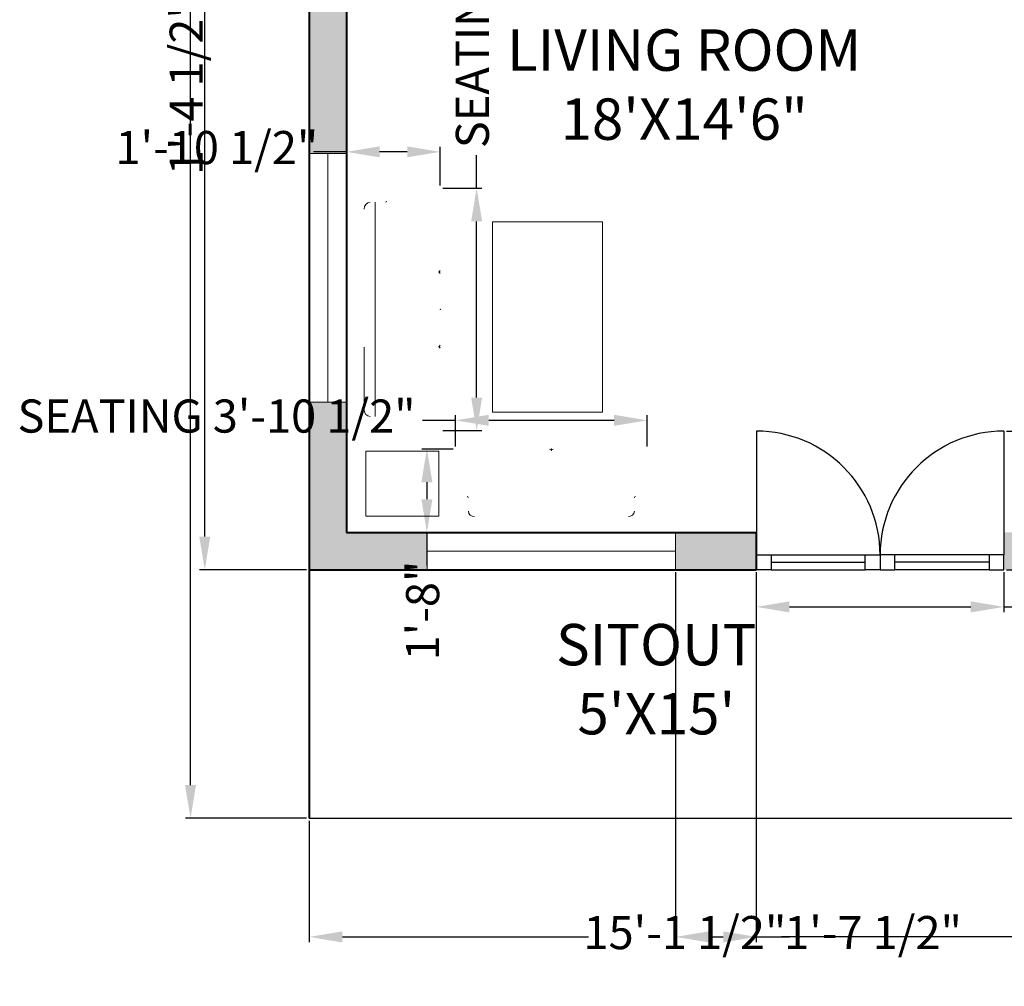
# Model space of a CAD drawing. Units: inches. Extents: x 2138 to 3265, y 2149 to 3392.
# Tile 1 of 13: x 2138 to 2375, y 2149 to 2382. Entities that reach past the tile are written whole.
import ezdxf

# ---------------------------------------------------------------- set-up
doc = ezdxf.new("R2010")
doc.units = ezdxf.units.IN
for name, color, linetype, lineweight in [('A-ANNO-DIMS', 2, 'Continuous', 18), ('A-AREA-IDEN', 7, 'Continuous', 18), ('A-DOOR', 22, 'Continuous', 25), ('A-FLOR', 7, 'Continuous', 25), ('A-FURN', 8, 'Continuous', 18), ('A-GLAZ', 150, 'Continuous', 18), ('A-WALL', 7, 'Continuous', 40), ('A-WALL-PATT', 142, 'Continuous', 13)]:
    doc.layers.add(name, color=color, linetype=linetype, lineweight=lineweight)
doc.styles.get("Standard").update_dxf_attribs({"font": 'arial.ttf'})
doc.dimstyles.new('ISO-25', dxfattribs={"dimtxt": 8, "dimasz": 8, "dimexe": 1.25, "dimexo": 0.625, "dimtad": 0, "dimdec": 1, "dimlunit": 4, "dimtxsty": 'Standard', "dimcen": 2.5, "dimadec": 0, "dimazin": 0, "dimtfac": 1, "dimtdec": 1, "dimtmove": 0, "dimatfit": 3, "dimfxl": 1, "dimarcsym": 0})

# ---------------------------------------------------------------- blocks, each defined once
blk = doc.blocks.new('Clinicians and patient chairs 13_dwgmodels.com')
at = {"color": 0}
for points in [[(-780.9, 0, 0, 0, 0), (-832.6, -11.1, 4.5, 4.5, 0)], [(-780.8, -0.7, 0, 0, 0), (-832.3, -11.8, 4.5, 4.5, 0)], [(-780.8, -0.7, 0, 0, 0), (-832.3, -11.8, 4.5, 4.5, 0)], [(780.9, 0, 0, 0, 0), (-780.9, 0, 4.5, 4.5, 0)], [(780.8, -0.7, 0, 0, 0), (-780.8, -0.7, 4.5, 4.5, 0)], [(780.8, -0.7, 0, 0, 0), (-780.8, -0.7, 4.5, 4.5, 0)], [(832.3, -11.8, 0, 0, 0), (780.8, -0.7, 4.5, 4.5, 0)], [(832.3, -11.8, 0, 0, 0), (780.8, -0.7, 4.5, 4.5, 0)], [(832.6, -11.1, 0, 0, 0), (780.9, 0, 4.5, 4.5, 0)], [(-888.6, -68.3, 0, 0, 0), (-898.5, -106.3, 4.5, 4.5, 0)], [(-888, -68.6, 0, 0, 0), (-897.8, -106.4, 4.5, 4.5, 0)], [(-867.7, -35.9, 0, 0, 0), (-888.6, -68.3, 4.5, 4.5, 0)], [(-867.1, -36.4, 0, 0, 0), (-888, -68.6, 4.5, 4.5, 0)], [(-867.1, -36.4, 0, 0, 0), (-888, -68.6, 4.5, 4.5, 0)], [(-872.1, -47.4, 0, 0, 0), (-872.1, -47.3, 4.5, 4.5, 0)], [(-832.6, -11.1, 0, 0, 0), (-867.7, -35.9, 4.5, 4.5, 0)], [(-832.3, -11.8, 0, 0, 0), (-867.1, -36.4, 4.5, 4.5, 0)], [(-832.3, -11.8, 0, 0, 0), (-867.1, -36.4, 4.5, 4.5, 0)], [(-854.1, -29.4, 0, 0, 0), (-854.1, -29.4, 4.5, 4.5, 0)], [(867.1, -36.4, 0, 0, 0), (832.3, -11.8, 4.5, 4.5, 0)], [(867.1, -36.4, 0, 0, 0), (832.3, -11.8, 4.5, 4.5, 0)], [(867.7, -35.9, 0, 0, 0), (832.6, -11.1, 4.5, 4.5, 0)], [(888, -68.6, 0, 0, 0), (867.1, -36.4, 4.5, 4.5, 0)], [(888, -68.6, 0, 0, 0), (867.1, -36.4, 4.5, 4.5, 0)], [(888.6, -68.3, 0, 0, 0), (867.7, -35.9, 4.5, 4.5, 0)], [(897.8, -106.4, 0, 0, 0), (888, -68.6, 4.5, 4.5, 0)], [(897.8, -106.4, 0, 0, 0), (888, -68.6, 4.5, 4.5, 0)], [(898.5, -106.3, 0, 0, 0), (888.6, -68.3, 4.5, 4.5, 0)], [(-898.5, -106.3, 0, 0, 0), (-898.5, -766.8, 4.5, 4.5, 0)], [(-897.8, -106.4, 0, 0, 0), (-897.8, -114.4, 4.5, 4.5, 0)], [(-897.8, -106.4, 0, 0, 0), (-897.8, -114.4, 4.5, 4.5, 0)], [(-897.8, -114.4, 0, 0, 0), (-897.8, -766.7, 4.5, 4.5, 0)], [(-897.8, -114.4, 0, 0, 0), (-897.8, -766.7, 4.5, 4.5, 0)], [(-897.8, -766.7, 0, 0, 0), (-897.8, -114.4, 4.5, 4.5, 0)], [(-896, -117.6, 0, 0, 0), (-896, -126.8, 4.5, 4.5, 0)], [(-896, -117.6, 0, 0, 0), (-896, -324.6, 4.5, 4.5, 0)], [(-896, -126.8, 0, 0, 0), (-896, -324.6, 4.5, 4.5, 0)], [(-22.2, -148.3, 0, 0, 0), (-722.5, -148.3, 4.5, 4.5, 0)], [(-8.3, -148.3, 0, 0, 0), (-22.2, -148.3, 4.5, 4.5, 0)], [(-8.3, -148.3, 0, 0, 0), (-7.7, -148.3, 4.5, 4.5, 0)], [(-7.7, -148.3, 0, 0, 0), (-6.2, -148.3, 4.5, 4.5, 0)], [(-6.2, -148.3, 0, 0, 0), (-1.3, -150.4, 4.5, 4.5, 0)], [(2.3, -149.9, 0, 0, 0), (-2.3, -149.9, 4.5, 4.5, 0)], [(-1.3, -150.4, 0, 0, 0), (0, -159.3, 4.5, 4.5, 0)], [(1.3, -150.4, 0, 0, 0), (0, -159.3, 4.5, 4.5, 0)], [(0, -159.3, 0, 0, 0), (0, -764.6, 4.5, 4.5, 0)], [(0, -159.3, 0, 0, 0), (0, -764.6, 4.5, 4.5, 0)], [(6.2, -148.3, 0, 0, 0), (1.3, -150.4, 4.5, 4.5, 0)], [(7.7, -148.3, 0, 0, 0), (6.2, -148.3, 4.5, 4.5, 0)], [(8.3, -148.3, 0, 0, 0), (7.7, -148.3, 4.5, 4.5, 0)], [(22.2, -148.3, 0, 0, 0), (8.3, -148.3, 4.5, 4.5, 0)], [(206.6, -148.3, 0, 0, 0), (22.2, -148.3, 4.5, 4.5, 0)], [(206.6, -148.3, 0, 0, 0), (722.5, -148.3, 4.5, 4.5, 0)], [(897.8, -114.4, 0, 0, 0), (897.8, -106.4, 4.5, 4.5, 0)], [(897.8, -114.4, 0, 0, 0), (897.8, -106.4, 4.5, 4.5, 0)], [(897.8, -766.7, 0, 0, 0), (897.8, -114.4, 4.5, 4.5, 0)], [(898.5, -766.8, 0, 0, 0), (898.5, -106.3, 4.5, 4.5, 0)], [(898.5, -766.8, 0, 0, 0), (898.5, -117.3, 4.5, 4.5, 0)], [(-896, -321.9, 0, 0, 0), (-896, -251.5, 4.5, 4.5, 0)], [(-779.6, -285, 0, 0, 0), (-779.4, -198.1, 4.5, 4.5, 0)], [(779.6, -285, 0, 0, 0), (779.4, -198.1, 4.5, 4.5, 0)], [(-896, -317.7, 0, 0, 0), (-896, -329.7, 4.5, 4.5, 0)], [(-896, -320.4, 0, 0, 0), (-896, -324.6, 4.5, 4.5, 0)], [(-896, -321.9, 0, 0, 0), (-896, -329.7, 4.5, 4.5, 0)], [(-896, -329.7, 0, 0, 0), (-896, -321.9, 4.5, 4.5, 0)], [(-896, -329.7, 0, 0, 0), (-892.2, -332.9, 4.5, 4.5, 0)], [(-892.2, -332.9, 0, 0, 0), (-892, -333, 4.5, 4.5, 0)], [(-892, -333, 0, 0, 0), (-891.9, -333.1, 4.5, 4.5, 0)], [(-886.9, -334.2, 0, 0, 0), (-891.9, -333.1, 4.5, 4.5, 0)], [(-886.9, -334.2, 0, 0, 0), (-837.4, -335.7, 4.5, 4.5, 0)], [(-837.4, -335.7, 0, 0, 0), (-790.1, -337, 4.5, 4.5, 0)], [(-779.8, -305.4, 0, 0, 0), (-779.9, -324.5, 4.5, 4.5, 0)], [(-779.6, -285, 0, 0, 0), (-779.8, -305.4, 4.5, 4.5, 0)], [(779.6, -285, 0, 0, 0), (779.8, -305.4, 4.5, 4.5, 0)], [(779.8, -305.4, 0, 0, 0), (779.9, -324.5, 4.5, 4.5, 0)], [(837.4, -335.7, 0, 0, 0), (790.1, -337, 4.5, 4.5, 0)], [(886.9, -334.2, 0, 0, 0), (837.4, -335.7, 4.5, 4.5, 0)], [(886.9, -334.2, 0, 0, 0), (891.9, -333.1, 4.5, 4.5, 0)], [(891.9, -333.1, 0, 0, 0), (892, -333, 4.5, 4.5, 0)], [(892.2, -332.9, 0, 0, 0), (892, -333, 4.5, 4.5, 0)], [(896, -329.7, 0, 0, 0), (892.2, -332.9, 4.5, 4.5, 0)], [(-898.5, -766.8, 0, 0, 0), (-895.2, -776, 4.5, 4.5, 0)], [(-895.2, -776, 0, 0, 0), (-898.5, -766.8, 4.5, 4.5, 0)], [(-897.8, -766.7, 0, 0, 0), (-894.5, -775.7, 4.5, 4.5, 0)], [(-897.8, -766.7, 0, 0, 0), (-894.5, -775.7, 4.5, 4.5, 0)], [(-894.5, -775.7, 0, 0, 0), (-897.8, -766.7, 4.5, 4.5, 0)], [(-894.5, -775.7, 0, 0, 0), (-897.8, -766.7, 4.5, 4.5, 0)], [(-895.2, -776, 0, 0, 0), (-894.6, -777.1, 4.5, 4.5, 0)], [(-894.6, -777.1, 0, 0, 0), (-895.2, -776, 4.5, 4.5, 0)], [(-894.5, -775.7, 0, 0, 0), (-894, -776.6, 4.5, 4.5, 0)], [(-894.5, -775.7, 0, 0, 0), (-894, -776.6, 4.5, 4.5, 0)], [(-894, -776.6, 0, 0, 0), (-894.5, -775.7, 4.5, 4.5, 0)], [(-894, -776.6, 0, 0, 0), (-894.5, -775.7, 4.5, 4.5, 0)], [(-894.6, -777.1, 0, 0, 0), (-893.6, -777.8, 4.5, 4.5, 0)], [(-893.6, -777.8, 0, 0, 0), (-894.6, -777.1, 4.5, 4.5, 0)], [(-894, -776.6, 0, 0, 0), (-893.2, -777.2, 4.5, 4.5, 0)], [(-894, -776.6, 0, 0, 0), (-893.2, -777.2, 4.5, 4.5, 0)], [(-893.2, -777.2, 0, 0, 0), (-894, -776.6, 4.5, 4.5, 0)], [(-893.2, -777.2, 0, 0, 0), (-894, -776.6, 4.5, 4.5, 0)], [(-893.6, -777.8, 0, 0, 0), (-886.6, -781, 4.5, 4.5, 0)], [(-886.6, -781, 0, 0, 0), (-893.6, -777.8, 4.5, 4.5, 0)], [(-893.2, -777.2, 0, 0, 0), (-886.5, -780.3, 4.5, 4.5, 0)], [(-893.2, -777.2, 0, 0, 0), (-886.5, -780.3, 4.5, 4.5, 0)], [(-886.5, -780.3, 0, 0, 0), (-893.2, -777.2, 4.5, 4.5, 0)], [(-886.5, -780.3, 0, 0, 0), (-893.2, -777.2, 4.5, 4.5, 0)], [(-886.6, -781, 0, 0, 0), (886.6, -781, 4.5, 4.5, 0)], [(886.6, -781, 0, 0, 0), (-886.6, -781, 4.5, 4.5, 0)], [(-886.5, -780.3, 0, 0, 0), (886.5, -780.3, 4.5, 4.5, 0)], [(-886.5, -780.3, 0, 0, 0), (886.5, -780.3, 4.5, 4.5, 0)], [(886.5, -780.3, 0, 0, 0), (-886.5, -780.3, 4.5, 4.5, 0)], [(886.5, -780.3, 0, 0, 0), (-886.5, -780.3, 4.5, 4.5, 0)], [(886.5, -780.3, 0, 0, 0), (893.2, -777.2, 4.5, 4.5, 0)], [(886.5, -780.3, 0, 0, 0), (893.2, -777.2, 4.5, 4.5, 0)], [(893.2, -777.2, 0, 0, 0), (886.5, -780.3, 4.5, 4.5, 0)], [(893.2, -777.2, 0, 0, 0), (886.5, -780.3, 4.5, 4.5, 0)], [(886.6, -781, 0, 0, 0), (893.6, -777.8, 4.5, 4.5, 0)], [(893.6, -777.8, 0, 0, 0), (886.6, -781, 4.5, 4.5, 0)], [(893.2, -777.2, 0, 0, 0), (894, -776.6, 4.5, 4.5, 0)], [(893.2, -777.2, 0, 0, 0), (894, -776.6, 4.5, 4.5, 0)], [(894, -776.6, 0, 0, 0), (893.2, -777.2, 4.5, 4.5, 0)], [(894, -776.6, 0, 0, 0), (893.2, -777.2, 4.5, 4.5, 0)], [(893.6, -777.8, 0, 0, 0), (894.6, -777.1, 4.5, 4.5, 0)], [(894.6, -777.1, 0, 0, 0), (893.6, -777.8, 4.5, 4.5, 0)], [(894.5, -775.7, 0, 0, 0), (894, -776.6, 4.5, 4.5, 0)], [(894.5, -775.7, 0, 0, 0), (894, -776.6, 4.5, 4.5, 0)], [(894.5, -775.7, 0, 0, 0), (894, -776.6, 4.5, 4.5, 0)], [(894.5, -775.7, 0, 0, 0), (894, -776.6, 4.5, 4.5, 0)], [(894.5, -775.7, 0, 0, 0), (897.8, -766.7, 4.5, 4.5, 0)], [(894.5, -775.7, 0, 0, 0), (897.8, -766.7, 4.5, 4.5, 0)], [(897.8, -766.7, 0, 0, 0), (894.5, -775.7, 4.5, 4.5, 0)], [(897.8, -766.7, 0, 0, 0), (894.5, -775.7, 4.5, 4.5, 0)], [(895.2, -776, 0, 0, 0), (894.6, -777.1, 4.5, 4.5, 0)], [(895.2, -776, 0, 0, 0), (894.6, -777.1, 4.5, 4.5, 0)], [(895.2, -776, 0, 0, 0), (898.5, -766.8, 4.5, 4.5, 0)], [(898.5, -766.8, 0, 0, 0), (895.2, -776, 4.5, 4.5, 0)]]:
    blk.add_lwpolyline(points, format="xyseb", dxfattribs=at)
for points in [[(-779.9, -324.5), (-779.9, -328.3)], [(779.9, -324.5), (779.9, -325.8)]]:
    blk.add_lwpolyline(points, dxfattribs=at)
for centre, radius, start, end in [((-724.7, -203.1), 54.9, 87.66786, 174.72548), ((724.7, -203.1), 54.9, 5.27444, 92.33206), ((-789.7, -327.1), 9.9, 267.95505, 352.93087), ((791.8, -325.1), 12, 183.2786, 261.48612), ((-17.2, -763), 17.3, 271.1045, 354.62389), ((17.2, -763), 17.3, 185.37611, 268.8955)]:
    blk.add_arc(centre, radius, start, end, dxfattribs=at)
blk.add_point((0, -781), dxfattribs=at)
blk = doc.blocks.new('Clinicians and patient chairs 9_dwgmodels.com')
at = {"color": 0}
for points in [[(-907.9, 0, 0, 0, 0), (-959.6, -11.1, 4.62, 4.62, 0)], [(907.9, 0, 0, 0, 0), (-907.9, 0, 4.62, 4.62, 0)], [(959.6, -11.1, 0, 0, 0), (907.9, 0, 4.62, 4.62, 0)], [(-1015.6, -68.3, 0, 0, 0), (-1025.5, -106.3, 4.62, 4.62, 0)], [(-994.7, -35.9, 0, 0, 0), (-1015.6, -68.3, 4.62, 4.62, 0)], [(-959.6, -11.1, 0, 0, 0), (-994.7, -35.9, 4.62, 4.62, 0)], [(994.7, -35.9, 0, 0, 0), (959.6, -11.1, 4.62, 4.62, 0)], [(1015.6, -68.3, 0, 0, 0), (994.7, -35.9, 4.62, 4.62, 0)], [(1025.5, -106.3, 0, 0, 0), (1015.6, -68.3, 4.62, 4.62, 0)], [(-1025.5, -106.3, 0, 0, 0), (-1025.5, -779.5, 4.62, 4.62, 0)], [(-313.4, -149.9, 0, 0, 0), (-318.1, -149.9, 4.62, 4.62, 0)], [(-314.5, -150.4, 0, 0, 0), (-315.7, -159.3, 4.62, 4.62, 0)], [(-315.7, -159.3, 0, 0, 0), (-315.7, -777.3, 4.62, 4.62, 0)], [(-309.5, -148.3, 0, 0, 0), (-314.5, -150.4, 4.62, 4.62, 0)], [(-308, -148.3, 0, 0, 0), (-309.5, -148.3, 4.62, 4.62, 0)], [(-307.5, -148.3, 0, 0, 0), (-308, -148.3, 4.62, 4.62, 0)], [(242.9, -148.3, 0, 0, 0), (-307.5, -148.3, 4.62, 4.62, 0)], [(242.9, -148.3, 0, 0, 0), (296, -148.3, 4.62, 4.62, 0)], [(296, -148.3, 0, 0, 0), (307.5, -148.3, 4.62, 4.62, 0)], [(308, -148.3, 0, 0, 0), (307.5, -148.3, 4.62, 4.62, 0)], [(309.5, -148.3, 0, 0, 0), (308, -148.3, 4.62, 4.62, 0)], [(309.5, -148.3, 0, 0, 0), (314.5, -150.4, 4.62, 4.62, 0)], [(849.5, -149.9, 0, 0, 0), (313.4, -149.9, 4.62, 4.62, 0)], [(314.5, -150.4, 0, 0, 0), (315.7, -159.3, 4.62, 4.62, 0)], [(315.7, -159.3, 0, 0, 0), (315.7, -777.3, 4.62, 4.62, 0)], [(315.7, -161.8, 0, 0, 0), (315.7, -777.3, 4.62, 4.62, 0)], [(1025.5, -779.5, 0, 0, 0), (1025.5, -106.3, 4.62, 4.62, 0)], [(1025.5, -779.5, 0, 0, 0), (1025.5, -117.3, 4.62, 4.62, 0)], [(-906.6, -285, 0, 0, 0), (-906.4, -198.1, 4.62, 4.62, 0)], [(906.9, -327, 0, 0, 0), (906.4, -199.7, 4.62, 4.62, 0)], [(-1023, -329.7, 0, 0, 0), (-1019.2, -332.9, 4.62, 4.62, 0)], [(-1019.2, -332.9, 0, 0, 0), (-1019, -333, 4.62, 4.62, 0)], [(-1019, -333, 0, 0, 0), (-1018.9, -333.1, 4.62, 4.62, 0)], [(-1013.9, -334.2, 0, 0, 0), (-1018.9, -333.1, 4.62, 4.62, 0)], [(-1013.9, -334.2, 0, 0, 0), (-964.4, -335.7, 4.62, 4.62, 0)], [(-906.8, -305.4, 0, 0, 0), (-906.9, -324.5, 4.62, 4.62, 0)], [(-906.9, -324.5, 0, 0, 0), (-906.9, -329.8, 4.62, 4.62, 0)], [(-906.6, -285, 0, 0, 0), (-906.8, -305.4, 4.62, 4.62, 0)], [(906.9, -327, 0, 0, 0), (906.9, -329.9, 4.62, 4.62, 0)], [(1013.9, -334.2, 0, 0, 0), (964.4, -335.7, 4.62, 4.62, 0)], [(1013.9, -334.2, 0, 0, 0), (1018.9, -333.1, 4.62, 4.62, 0)], [(1018.9, -333.1, 0, 0, 0), (1019, -333, 4.62, 4.62, 0)], [(1019.2, -332.9, 0, 0, 0), (1019, -333, 4.62, 4.62, 0)], [(1023, -329.7, 0, 0, 0), (1019.2, -332.9, 4.62, 4.62, 0)], [(-1019.8, -340.2, 0, 0, 0), (-1023, -348.6, 4.62, 4.62, 0)], [(-1010.3, -335.9, 0, 0, 0), (-1019.8, -340.2, 4.62, 4.62, 0)], [(-917.1, -337, 0, 0, 0), (-1010.3, -335.9, 4.62, 4.62, 0)], [(-964.4, -335.7, 0, 0, 0), (-927.1, -336.8, 4.62, 4.62, 0)], [(964.4, -335.7, 0, 0, 0), (914.9, -337.2, 4.62, 4.62, 0)], [(917.1, -339.4, 0, 0, 0), (1010.3, -338.4, 4.62, 4.62, 0)], [(1010.3, -338.4, 0, 0, 0), (1019.8, -342.7, 4.62, 4.62, 0)], [(1019.8, -342.7, 0, 0, 0), (1023, -351.1, 4.62, 4.62, 0)], [(1023, -351.1, 0, 0, 0), (1022.6, -779.8, 4.62, 4.62, 0)], [(-1025.5, -779.5, 0, 0, 0), (-1022.2, -788.7, 4.62, 4.62, 0)], [(-1022.2, -788.7, 0, 0, 0), (-1021.6, -789.8, 4.62, 4.62, 0)], [(-1021.6, -789.8, 0, 0, 0), (-1020.6, -790.5, 4.62, 4.62, 0)], [(-1020.6, -790.5, 0, 0, 0), (-1013.6, -793.7, 4.62, 4.62, 0)], [(-1013.6, -793.7, 0, 0, 0), (1013.6, -793.7, 4.62, 4.62, 0)], [(1019.8, -788.8, 0, 0, 0), (1013.1, -793.7, 4.62, 4.62, 0)], [(1013.6, -793.7, 0, 0, 0), (1020.6, -790.5, 4.62, 4.62, 0)], [(1022.6, -779.8, 0, 0, 0), (1019.8, -788.8, 4.62, 4.62, 0)], [(1020.6, -790.5, 0, 0, 0), (1021.6, -789.8, 4.62, 4.62, 0)], [(1022.2, -788.7, 0, 0, 0), (1021.6, -789.8, 4.62, 4.62, 0)], [(1022.2, -788.7, 0, 0, 0), (1025.5, -779.5, 4.62, 4.62, 0)]]:
    blk.add_lwpolyline(points, format="xyseb", dxfattribs=at)
for points in [[(-849.5, -149.9), (-318.1, -149.9)], [(-906.5, -241.5), (906.5, -242.3)]]:
    blk.add_lwpolyline(points, dxfattribs=at)
for centre, radius, start, end in [((-851.7, -204.8), 54.9, 87.66794, 174.72556), ((851.7, -204.8), 54.9, 5.27444, 92.33206), ((-916.6, -326.8), 10.2, 267.54544, 342.40568), ((916.9, -329.4), 10, 182.60942, 270.79497), ((-337, -773.8), 21.5, 292.11503, 350.63044), ((-294.5, -773.8), 21.5, 189.36956, 247.88497), ((294.5, -773.8), 21.5, 292.11503, 350.63044), ((336.9, -773.8), 21.5, 189.36956, 247.88497)]:
    blk.add_arc(centre, radius, start, end, dxfattribs=at)
blk.add_point((0, -793.7), dxfattribs=at)
blk = doc.blocks.new('d')
for points in [[(1948.9, 2369.07), (1948.9, 2346.04)], [(1994.96, 2369.07), (1994.96, 2346.04)], [(1951.65, 2346.04), (1969.17, 2346.04)], [(1992.2, 2346.04), (1974.69, 2346.04)], [(1951.65, 2344.66), (1969.17, 2344.66)], [(1951.65, 2343.29), (1969.17, 2343.29)], [(1992.2, 2344.66), (1974.69, 2344.66)], [(1992.2, 2343.29), (1974.69, 2343.29)]]:
    blk.add_lwpolyline(points)
for points in [[(1948.9, 2346.04), (1951.65, 2346.04), (1951.65, 2343.29), (1948.9, 2343.29)], [(1969.17, 2346.04), (1971.93, 2346.04), (1971.93, 2343.29), (1969.17, 2343.29)], [(1969.17, 2346.04), (1971.93, 2346.04), (1971.93, 2343.29), (1969.17, 2343.29)], [(1974.69, 2346.04), (1971.93, 2346.04), (1971.93, 2343.29), (1974.69, 2343.29)], [(1994.96, 2346.04), (1992.2, 2346.04), (1992.2, 2343.29), (1994.96, 2343.29)]]:
    blk.add_lwpolyline(points, close=True)
for centre, start, end in [((1948.9, 2346.04), 0, 90), ((1994.96, 2346.04), 90, 180)]:
    blk.add_arc(centre, 23.03, start, end)
blk = doc.blocks.new('*D19')
at = {"layer": 'A-ANNO-DIMS', "color": 0, "lineweight": -2, "transparency": 16777216}
for p, q in [((2206.9, 2729.66), (2181.05, 2729.66)), ((2182.3, 2721.66), (2182.3, 2497.24)), ((2182.3, 2257.66), (2182.3, 2482.09)), ((2206.9, 2249.66), (2181.05, 2249.66))]:
    blk.add_line(p, q, dxfattribs=at)
at = {"layer": 'A-ANNO-DIMS', "color": 0, "transparency": 16777216}
for points in [[(2180.97, 2721.66), (2183.63, 2721.66), (2182.3, 2729.66)], [(2180.97, 2257.66), (2183.63, 2257.66), (2182.3, 2249.66)]]:
    blk.add_solid(points, dxfattribs=at)
at = {"layer": 'Defpoints', "color": 0, "transparency": 16777216}
for p in [(2207.53, 2729.66), (2182.3, 2249.66), (2207.53, 2249.66)]:
    blk.add_point(p, dxfattribs=at)
at = {"layer": 'A-ANNO-DIMS', "color": 0, "transparency": 16777216, "insert": (2182.3, 2489.66), "char_height": 8, "attachment_point": 5, "rotation": 90}
blk.add_mtext("40'", dxfattribs=at)
blk = doc.blocks.new('GLAZ-SASH-60IN')
for p, q in [((0, 9), (0, 0)), ((60, 9), (60, 0)), ((0, 4.5), (60, 4.5))]:
    blk.add_line(p, q)
blk = doc.blocks.new('*D31')
at = {"layer": 'A-ANNO-DIMS', "color": 0, "lineweight": -2, "transparency": 16777216}
for p, q in [((2315.53, 2249.04), (2315.53, 2239.44)), ((2375.34, 2249.04), (2375.34, 2239.44)), ((2323.53, 2240.69), (2367.34, 2240.69)), ((2375.34, 2240.69), (2383.34, 2240.69))]:
    blk.add_line(p, q, dxfattribs=at)
at = {"layer": 'A-ANNO-DIMS', "color": 0, "transparency": 16777216}
for points in [[(2323.53, 2242.02), (2323.53, 2239.36), (2315.53, 2240.69)], [(2367.34, 2242.02), (2367.34, 2239.36), (2375.34, 2240.69)]]:
    blk.add_solid(points, dxfattribs=at)
at = {"layer": 'Defpoints', "color": 0, "transparency": 16777216}
for p in [(2315.53, 2249.66), (2375.34, 2249.66), (2375.34, 2240.69)]:
    blk.add_point(p, dxfattribs=at)
at = {"layer": 'A-ANNO-DIMS', "color": 0, "transparency": 16777216, "insert": (2433.19, 2240.69), "char_height": 8, "attachment_point": 5}
blk.add_mtext('ENTRY DOOR 5\'-0"', dxfattribs=at)
blk = doc.blocks.new('*D32')
at = {"layer": 'A-ANNO-DIMS', "color": 0, "lineweight": -2, "transparency": 16777216}
for p, q in [((2384.31, 2283.14), (2384.31, 2291.14)), ((2375.96, 2283.14), (2385.56, 2283.14)), ((2384.31, 2257.66), (2384.31, 2275.14)), ((2375.96, 2249.66), (2385.56, 2249.66))]:
    blk.add_line(p, q, dxfattribs=at)
at = {"layer": 'A-ANNO-DIMS', "color": 0, "transparency": 16777216}
for points in [[(2382.97, 2275.14), (2385.64, 2275.14), (2384.31, 2283.14)], [(2382.97, 2257.66), (2385.64, 2257.66), (2384.31, 2249.66)]]:
    blk.add_solid(points, dxfattribs=at)
at = {"layer": 'Defpoints', "color": 0, "transparency": 16777216}
for p in [(2375.34, 2283.14), (2384.31, 2283.14), (2375.34, 2249.66)]:
    blk.add_point(p, dxfattribs=at)
at = {"layer": 'A-ANNO-DIMS', "color": 0, "transparency": 16777216, "insert": (2384.31, 2311.79), "char_height": 8, "attachment_point": 5, "rotation": 90}
blk.add_mtext('2\'-9 1/2"', dxfattribs=at)
blk = doc.blocks.new('*D39')
at = {"layer": 'A-ANNO-DIMS', "color": 0, "lineweight": -2, "transparency": 16777216}
for p, q in [((2242.89, 2285.74), (2234.89, 2285.74)), ((2242.89, 2279.43), (2242.89, 2286.99)), ((2281.17, 2285.74), (2250.89, 2285.74)), ((2289.17, 2279.43), (2289.17, 2286.99))]:
    blk.add_line(p, q, dxfattribs=at)
at = {"layer": 'A-ANNO-DIMS', "color": 0, "transparency": 16777216}
for points in [[(2250.89, 2287.08), (2250.89, 2284.41), (2242.89, 2285.74)], [(2281.17, 2287.08), (2281.17, 2284.41), (2289.17, 2285.74)]]:
    blk.add_solid(points, dxfattribs=at)
at = {"layer": 'Defpoints', "color": 0, "transparency": 16777216}
for p in [(2242.89, 2285.74), (2242.89, 2278.8), (2289.17, 2278.8)]:
    blk.add_point(p, dxfattribs=at)
at = {"layer": 'A-ANNO-DIMS', "color": 0, "transparency": 16777216, "insert": (2185.14, 2285.74), "char_height": 8, "attachment_point": 5}
blk.add_mtext('SEATING 3\'-10 1/2"', dxfattribs=at)
blk = doc.blocks.new('*D40')
at = {"layer": 'A-ANNO-DIMS', "color": 0, "lineweight": -2, "transparency": 16777216}
for p, q in [((2242.27, 2278.8), (2234.7, 2278.8)), ((2235.95, 2270.8), (2235.95, 2266.69)), ((2242.27, 2258.69), (2234.7, 2258.69)), ((2235.95, 2258.69), (2235.95, 2250.69))]:
    blk.add_line(p, q, dxfattribs=at)
at = {"layer": 'A-ANNO-DIMS', "color": 0, "transparency": 16777216}
for points in [[(2234.62, 2270.8), (2237.28, 2270.8), (2235.95, 2278.8)], [(2234.62, 2266.69), (2237.28, 2266.69), (2235.95, 2258.69)]]:
    blk.add_solid(points, dxfattribs=at)
at = {"layer": 'Defpoints', "color": 0, "transparency": 16777216}
for p in [(2242.89, 2278.8), (2235.95, 2258.69), (2242.89, 2258.69)]:
    blk.add_point(p, dxfattribs=at)
at = {"layer": 'A-ANNO-DIMS', "color": 0, "transparency": 16777216, "insert": (2235.95, 2239.81), "char_height": 8, "attachment_point": 5, "rotation": 90}
blk.add_mtext('1\'-8"', dxfattribs=at)
blk = doc.blocks.new('*D41')
at = {"layer": 'A-ANNO-DIMS', "color": 0, "lineweight": -2, "transparency": 16777216}
for p, q in [((2247.97, 2341.8), (2247.97, 2349.8)), ((2239.81, 2341.8), (2249.22, 2341.8)), ((2247.97, 2291.25), (2247.97, 2333.8)), ((2239.81, 2283.25), (2249.22, 2283.25))]:
    blk.add_line(p, q, dxfattribs=at)
at = {"layer": 'A-ANNO-DIMS', "color": 0, "transparency": 16777216}
for points in [[(2246.64, 2333.8), (2249.3, 2333.8), (2247.97, 2341.8)], [(2246.64, 2291.25), (2249.3, 2291.25), (2247.97, 2283.25)]]:
    blk.add_solid(points, dxfattribs=at)
at = {"layer": 'Defpoints', "color": 0, "transparency": 16777216}
for p in [(2239.19, 2341.8), (2247.97, 2341.8), (2239.19, 2283.25)]:
    blk.add_point(p, dxfattribs=at)
at = {"layer": 'A-ANNO-DIMS', "color": 0, "transparency": 16777216, "insert": (2247.97, 2399.55), "char_height": 8, "attachment_point": 5, "rotation": 90}
blk.add_mtext('SEATING 4\'-10 1/2"', dxfattribs=at)
blk = doc.blocks.new('*D42')
at = {"layer": 'A-ANNO-DIMS', "color": 0, "lineweight": -2, "transparency": 16777216}
for p, q in [((2216.53, 2350.58), (2208.53, 2350.58)), ((2216.53, 2342.42), (2216.53, 2351.83)), ((2231.19, 2350.58), (2224.53, 2350.58)), ((2239.19, 2342.42), (2239.19, 2351.83))]:
    blk.add_line(p, q, dxfattribs=at)
at = {"layer": 'A-ANNO-DIMS', "color": 0, "transparency": 16777216}
for points in [[(2224.53, 2351.91), (2224.53, 2349.25), (2216.53, 2350.58)], [(2231.19, 2351.91), (2231.19, 2349.25), (2239.19, 2350.58)]]:
    blk.add_solid(points, dxfattribs=at)
at = {"layer": 'Defpoints', "color": 0, "transparency": 16777216}
for p in [(2216.53, 2350.58), (2216.53, 2341.8), (2239.19, 2341.8)]:
    blk.add_point(p, dxfattribs=at)
at = {"layer": 'A-ANNO-DIMS', "color": 0, "transparency": 16777216, "insert": (2185.22, 2350.58), "char_height": 8, "attachment_point": 5}
blk.add_mtext('1\'-10 1/2"', dxfattribs=at)
blk = doc.blocks.new('*D51')
at = {"layer": 'A-ANNO-DIMS', "color": 0, "lineweight": -2, "transparency": 16777216}
for p, q in [((2206.9, 2729.66), (2177.6, 2729.66)), ((2178.85, 2721.66), (2178.85, 2474.19)), ((2178.85, 2197.66), (2178.85, 2445.13)), ((2206.9, 2189.66), (2177.6, 2189.66))]:
    blk.add_line(p, q, dxfattribs=at)
at = {"layer": 'A-ANNO-DIMS', "color": 0, "transparency": 16777216}
for points in [[(2177.52, 2721.66), (2180.19, 2721.66), (2178.85, 2729.66)], [(2177.52, 2197.66), (2180.19, 2197.66), (2178.85, 2189.66)]]:
    blk.add_solid(points, dxfattribs=at)
at = {"layer": 'Defpoints', "color": 0, "transparency": 16777216}
for p in [(2178.85, 2729.66), (2207.53, 2729.66), (2207.53, 2189.66)]:
    blk.add_point(p, dxfattribs=at)
at = {"layer": 'A-ANNO-DIMS', "color": 0, "transparency": 16777216, "insert": (2178.85, 2459.66), "char_height": 8, "attachment_point": 5, "rotation": 90}
blk.add_mtext('45\'-0"', dxfattribs=at)
blk = doc.blocks.new('*D52')
at = {"layer": 'A-ANNO-DIMS', "color": 0, "lineweight": -2, "transparency": 16777216}
for p, q in [((2207.53, 2189.04), (2207.53, 2159.74)), ((2389.03, 2189.04), (2389.03, 2159.74)), ((2215.53, 2160.99), (2274.97, 2160.99)), ((2381.03, 2160.99), (2321.59, 2160.99))]:
    blk.add_line(p, q, dxfattribs=at)
at = {"layer": 'A-ANNO-DIMS', "color": 0, "transparency": 16777216}
for points in [[(2215.53, 2162.32), (2215.53, 2159.65), (2207.53, 2160.99)], [(2381.03, 2162.32), (2381.03, 2159.65), (2389.03, 2160.99)]]:
    blk.add_solid(points, dxfattribs=at)
at = {"layer": 'Defpoints', "color": 0, "transparency": 16777216}
for p in [(2207.53, 2189.66), (2389.03, 2189.66), (2389.03, 2160.99)]:
    blk.add_point(p, dxfattribs=at)
at = {"layer": 'A-ANNO-DIMS', "color": 0, "transparency": 16777216, "insert": (2298.28, 2160.99), "char_height": 8, "attachment_point": 5}
blk.add_mtext('15\'-1 1/2"', dxfattribs=at)
blk = doc.blocks.new('*D59')
at = {"layer": 'A-ANNO-DIMS', "color": 0, "lineweight": -2, "transparency": 16777216}
for p, q in [((2296.03, 2249.04), (2296.03, 2159.74)), ((2315.53, 2249.04), (2315.53, 2159.74)), ((2304.03, 2160.99), (2307.53, 2160.99)), ((2315.53, 2160.99), (2323.53, 2160.99))]:
    blk.add_line(p, q, dxfattribs=at)
at = {"layer": 'A-ANNO-DIMS', "color": 0, "transparency": 16777216}
for points in [[(2304.03, 2162.32), (2304.03, 2159.65), (2296.03, 2160.99)], [(2307.53, 2162.32), (2307.53, 2159.65), (2315.53, 2160.99)]]:
    blk.add_solid(points, dxfattribs=at)
at = {"layer": 'Defpoints', "color": 0, "transparency": 16777216}
for p in [(2296.03, 2249.66), (2315.53, 2249.66), (2315.53, 2160.99)]:
    blk.add_point(p, dxfattribs=at)
at = {"layer": 'A-ANNO-DIMS', "color": 0, "transparency": 16777216, "insert": (2343.73, 2160.99), "char_height": 8, "attachment_point": 5}
blk.add_mtext('1\'-7 1/2"', dxfattribs=at)
blk = doc.blocks.new('*D60')
at = {"layer": 'A-ANNO-DIMS', "color": 0, "lineweight": -2, "transparency": 16777216}
for p, q in [((2178.85, 2427.16), (2178.85, 2435.16)), ((2493.4, 2419.16), (2177.6, 2419.16)), ((2178.85, 2419.16), (2178.85, 2402.66)), ((2493.4, 2402.66), (2177.6, 2402.66)), ((2178.85, 2394.66), (2178.85, 2386.66))]:
    blk.add_line(p, q, dxfattribs=at)
at = {"layer": 'A-ANNO-DIMS', "color": 0, "transparency": 16777216}
for points in [[(2177.52, 2427.16), (2180.19, 2427.16), (2178.85, 2419.16)], [(2177.52, 2394.66), (2180.19, 2394.66), (2178.85, 2402.66)]]:
    blk.add_solid(points, dxfattribs=at)
at = {"layer": 'Defpoints', "color": 0, "transparency": 16777216}
for p in [(2494.03, 2419.16), (2178.85, 2402.66), (2494.03, 2402.66)]:
    blk.add_point(p, dxfattribs=at)
at = {"layer": 'A-ANNO-DIMS', "color": 0, "transparency": 16777216, "insert": (2178.85, 2366.46), "char_height": 8, "attachment_point": 5, "rotation": 90}
blk.add_mtext('1\'-4 1/2"', dxfattribs=at)

msp = doc.modelspace()

# ---------------------------------------------------------------- hatches: boundary and pattern name
at = {"layer": 'A-WALL-PATT'}
h = msp.add_hatch(color=256, dxfattribs=at)
h.dxf.hatch_style = 1
h.paths.add_polyline_path([(2270.53, 2729.66), (2207.53, 2729.66), (2207.53, 2663.66), (2216.53, 2663.66), (2216.53, 2720.66), (2270.53, 2720.66)])
h.paths.add_polyline_path([(2484.36, 2729.66), (2330.53, 2729.66), (2330.53, 2720.66), (2384.53, 2720.66), (2384.53, 2546.66), (2372.53, 2546.66), (2372.53, 2542.16), (2389.03, 2542.16), (2389.03, 2720.66), (2484.36, 2720.66)])
h.paths.add_polyline_path([(2591.53, 2729.66), (2544.36, 2729.66), (2544.36, 2720.66), (2582.53, 2720.66), (2582.53, 2684.66), (2591.53, 2684.66)])
h.paths.add_polyline_path([(2591.53, 2624.66), (2582.53, 2624.66), (2582.53, 2588.66), (2456.53, 2588.66), (2456.53, 2584.16), (2582.53, 2584.16), (2582.53, 2512.16), (2456.53, 2512.16), (2456.53, 2507.66), (2494.03, 2507.66), (2494.03, 2501.66), (2498.53, 2501.66), (2498.53, 2507.66), (2582.53, 2507.66), (2582.53, 2495.66), (2591.53, 2495.66)])
h.paths.add_polyline_path([(2591.53, 2471.66), (2582.53, 2471.66), (2582.53, 2459.66), (2498.53, 2459.66), (2498.53, 2471.66), (2497.72, 2471.66, -0.030629), (2494.03, 2471.44), (2494.03, 2459.66), (2431.08, 2459.66, -0.013128), (2431.03, 2457.77), (2431.03, 2455.16), (2494.03, 2455.16), (2494.03, 2449.16), (2498.53, 2449.16), (2498.53, 2455.16), (2582.53, 2455.16), (2582.53, 2443.16), (2591.53, 2443.16)])
h.paths.add_polyline_path([(2591.53, 2419.16), (2582.53, 2419.16), (2582.53, 2407.16), (2498.53, 2407.16), (2498.53, 2419.16), (2497.72, 2419.16, -0.030629), (2494.03, 2418.94), (2494.03, 2402.66), (2582.53, 2402.66), (2582.53, 2360.66), (2591.53, 2360.66)])
h.paths.add_polyline_path([(2591.53, 2300.66), (2582.53, 2300.66), (2582.53, 2258.66), (2515.78, 2258.66), (2515.78, 2249.66), (2591.53, 2249.66)])
h.paths.add_polyline_path([(2455.78, 2258.66), (2389.03, 2258.66), (2389.03, 2455.16), (2395.03, 2455.16), (2395.03, 2459.66), (2384.53, 2459.66), (2384.53, 2258.66), (2375.53, 2258.66), (2375.53, 2249.66), (2455.78, 2249.66)])
h.paths.add_polyline_path([(2315.53, 2253.24), (2315.53, 2258.66), (2296.03, 2258.66), (2296.03, 2249.66), (2315.53, 2249.66)])
h.paths.add_polyline_path([(2236.03, 2258.66), (2216.53, 2258.66), (2216.53, 2290.16), (2207.53, 2290.16), (2207.53, 2249.66), (2236.03, 2249.66)])
h.paths.add_polyline_path([(2216.53, 2396.66), (2207.53, 2396.66), (2207.53, 2350.16), (2216.53, 2350.16)])
h.paths.add_polyline_path([(2216.53, 2603.66), (2207.53, 2603.66), (2207.53, 2456.66), (2216.53, 2456.66), (2216.53, 2542.16), (2264.53, 2542.16), (2264.53, 2470.16), (2252.53, 2470.16), (2252.53, 2465.66), (2269.03, 2465.66), (2269.03, 2542.16), (2336.48, 2542.16, -0.013128), (2336.53, 2544.05), (2336.53, 2546.66), (2216.53, 2546.66)])

# ---------------------------------------------------------------- linework, layer by layer
at = {"layer": 'A-FLOR'}
msp.add_line((2207.53, 2189.66), (2389.03, 2189.66), dxfattribs=at)
at = {"layer": 'A-FURN'}
for points in [[(2251.77, 2333.72), (2278.37, 2333.72), (2278.37, 2287.74), (2251.77, 2287.74)], [(2221.2, 2278.31), (2238.87, 2278.31), (2238.87, 2262.59), (2221.2, 2262.59)]]:
    msp.add_lwpolyline(points, close=True, dxfattribs=at)
at = {"layer": 'A-GLAZ'}
for points in [[(2207.53, 2350.16), (2216.53, 2350.16), (2216.53, 2290.16), (2207.53, 2290.16)], [(2236.03, 2258.66), (2296.03, 2258.66), (2296.03, 2249.66), (2236.03, 2249.66)]]:
    msp.add_lwpolyline(points, close=True, dxfattribs=at)
at = {"layer": 'A-WALL'}
for p, q in [((2207.53, 2729.66), (2207.53, 2189.66)), ((2216.53, 2456.66), (2216.53, 2258.66)), ((2216.53, 2258.66), (2315.53, 2258.66)), ((2315.53, 2258.66), (2315.53, 2249.66)), ((2207.53, 2249.66), (2315.53, 2249.66))]:
    msp.add_line(p, q, dxfattribs=at)

# ---------------------------------------------------------------- block references
at = {"layer": 'A-DOOR', "xscale": 1.29834981914095, "yscale": 1.29834981914095, "zscale": 1.29834981914095}
msp.add_blockref('d', (-214.82, -792.74), dxfattribs=at)
at = {"layer": 'A-FURN'}
for name, p, xscale, yscale, zscale, rotation in [('Clinicians and patient chairs 9_dwgmodels.com', (2216.53, 2312.53), 0.0285453031443639, 0.0285453031443639, 0.0285453031443639, 90), ('Clinicians and patient chairs 13_dwgmodels.com', (2266.03, 2258.69), 0.0257501154052157, 0.0257501154052157, 0.0257501154052157, 180)]:
    msp.add_blockref(name, p, dxfattribs=dict(at, xscale=xscale, yscale=yscale, zscale=zscale, rotation=rotation))
at = {"layer": 'A-GLAZ', "rotation": 89.9999999999994}
msp.add_blockref('GLAZ-SASH-60IN', (2216.53, 2290.16), dxfattribs=at)
at = {"layer": 'A-GLAZ'}
msp.add_blockref('GLAZ-SASH-60IN', (2236.03, 2249.66), dxfattribs=at)

# ---------------------------------------------------------------- texts
at = {"layer": 'A-AREA-IDEN', "char_height": 10, "attachment_point": 1}
for s, width, insert in [('\\pxqc;LIVING ROOM\\P18\'X14\'6"', 102.811, (2246.7, 2380.16)), ("\\pxqc;SITOUT\\P5'X15'", 77.0226, (2252.86, 2236.57))]:
    msp.add_mtext_dynamic_manual_height_columns(s, width=width, gutter_width=12.5, heights=[0], dxfattribs=dict(at, insert=insert))

# ---------------------------------------------------------------- dimensions: what is measured, and where the dimension line sits
at = {"layer": 'A-ANNO-DIMS'}
for base, p1, p2, angle, override, picture, middle in [((2178.85, 2729.66), (2207.53, 2189.66), (2207.53, 2729.66), 90, {"dimdec": 1, "dimlfac": 1, "dimrnd": 0, "dimzin": 1, "dimdsep": 46, "dimlunit": 4, "dimfrac": 2}, '*D51', (2178.85, 2459.66)), ((2182.3, 2249.66), (2207.53, 2729.66), (2207.53, 2249.66), 90, {"dimclrd": 0, "dimclre": 0, "dimclrt": 0}, '*D19', (2182.3, 2489.66)), ((2178.85, 2402.66), (2494.03, 2419.16), (2494.03, 2402.66), 90, {"dimdec": 1, "dimlfac": 1, "dimrnd": 0, "dimzin": 1, "dimdsep": 46, "dimlunit": 4, "dimfrac": 2}, '*D60', (2178.85, 2366.46)), ((2216.53, 2350.58), (2239.19, 2341.8), (2216.53, 2341.8), 180, {"dimdec": 1, "dimlfac": 1, "dimrnd": 0, "dimzin": 1, "dimdsep": 46, "dimlunit": 4, "dimfrac": 2}, '*D42', (2185.22, 2350.58)), ((2384.31, 2283.14), (2375.34, 2249.66), (2375.34, 2283.14), 90, {"dimdec": 1, "dimlfac": 1, "dimrnd": 0, "dimzin": 1, "dimdsep": 46, "dimlunit": 4, "dimfrac": 2}, '*D32', (2384.31, 2311.79)), ((2235.95, 2258.69), (2242.89, 2278.8), (2242.89, 2258.69), 270, {"dimdec": 1, "dimlfac": 1, "dimrnd": 0, "dimzin": 1, "dimdsep": 46, "dimlunit": 4, "dimfrac": 2}, '*D40', (2235.95, 2239.81))]:
    dim = msp.add_linear_dim(base=base, p1=p1, p2=p2, angle=angle, dimstyle='ISO-25', override=override, dxfattribs=at)
    dim.commit()
    dim.dimension.update_dxf_attribs({"geometry": picture, "text_midpoint": middle})
for base, p1, p2, angle, picture, middle in [((2247.9691, 2341.7994), (2239.187, 2283.2518), (2239.187, 2341.7994), 90, '*D41', (2247.9691, 2399.5485)), ((2242.89, 2285.74), (2289.17, 2278.8), (2242.89, 2278.8), 180, '*D39', (2185.14, 2285.74))]:
    dim = msp.add_linear_dim(base=base, p1=p1, p2=p2, angle=angle, text='SEATING <>', dimstyle='ISO-25', override={"dimdec": 1, "dimlfac": 1, "dimrnd": 0, "dimzin": 1, "dimdsep": 46, "dimlunit": 4, "dimfrac": 2}, dxfattribs=at)
    dim.commit()
    dim.dimension.update_dxf_attribs({"geometry": picture, "text_midpoint": middle})
dim = msp.add_linear_dim(base=(2375.34, 2240.69), p1=(2315.53, 2249.66), p2=(2375.34, 2249.66), text='ENTRY DOOR <>', dimstyle='ISO-25', override={"dimdec": 1, "dimlfac": 1, "dimrnd": 0, "dimzin": 1, "dimdsep": 46, "dimlunit": 4, "dimfrac": 2}, dxfattribs=at)
dim.commit()
dim.dimension.update_dxf_attribs({"geometry": '*D31', "text_midpoint": (2433.19, 2240.69)})
for base, p1, p2, picture, middle in [((2315.53, 2160.99), (2296.03, 2249.66), (2315.53, 2249.66), '*D59', (2343.73, 2160.99)), ((2389.03, 2160.99), (2207.53, 2189.66), (2389.03, 2189.66), '*D52', (2298.28, 2160.99))]:
    dim = msp.add_linear_dim(base=base, p1=p1, p2=p2, dimstyle='ISO-25', override={"dimdec": 1, "dimlfac": 1, "dimrnd": 0, "dimzin": 1, "dimdsep": 46, "dimlunit": 4, "dimfrac": 2}, dxfattribs=at)
    dim.commit()
    dim.dimension.update_dxf_attribs({"geometry": picture, "text_midpoint": middle})

doc.saveas('drawing.dxf')
